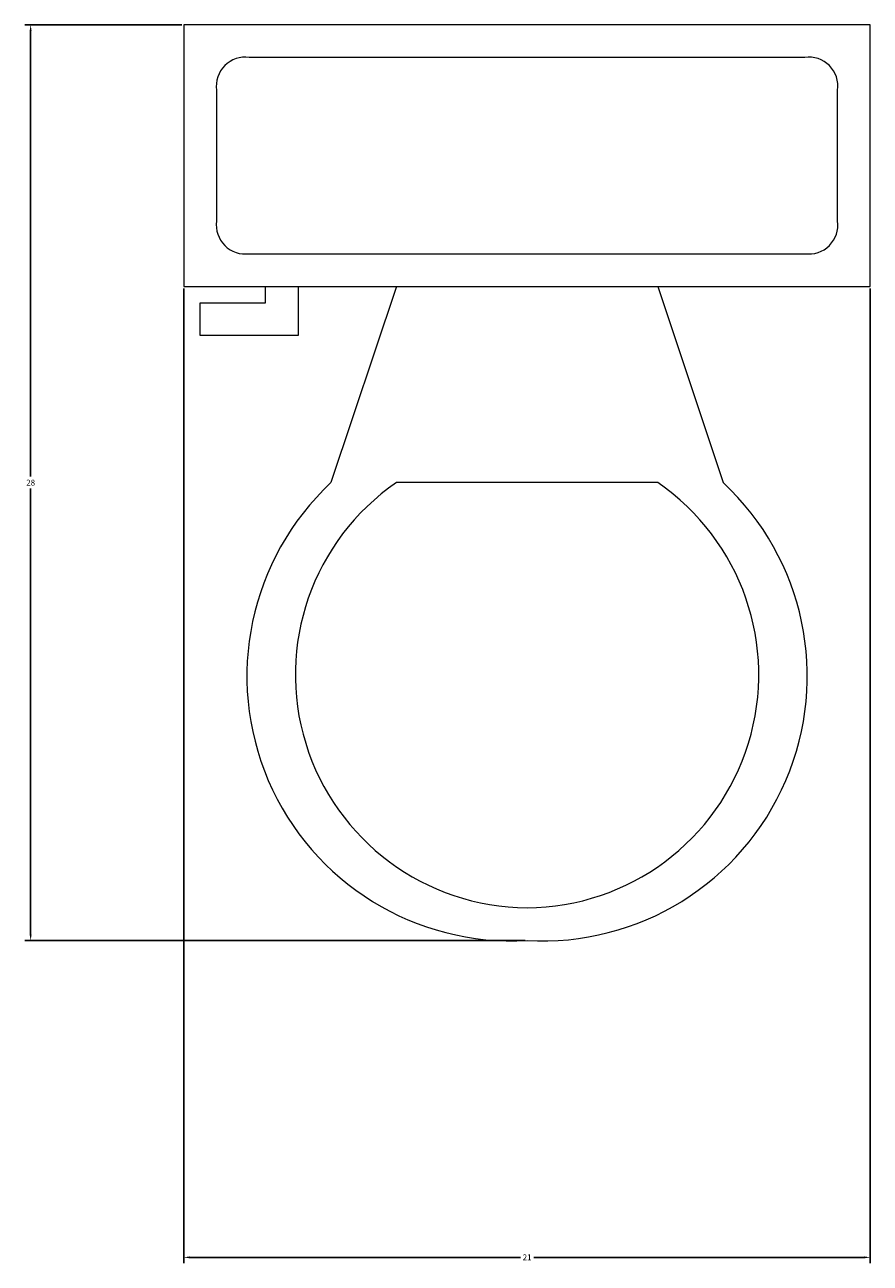
# Model space of a CAD drawing. Units: inches. Extents: x 2070 to 4408, y 1595 to 4269.
# Tile 20 of 20: x 4382 to 4408, y 4231 to 4269. Entities that reach past the tile are written whole.
import ezdxf

# ---------------------------------------------------------------- set-up
doc = ezdxf.new("R2010")
doc.units = ezdxf.units.IN
doc.layers.add('A-ANNO-DIMS', color=2, linetype='Continuous', lineweight=18)
doc.layers.add('A-FLOR-FIXT', color=9, linetype='Continuous', lineweight=18)
doc.styles.get("Standard").update_dxf_attribs({"font": 'arial.ttf'})
doc.dimstyles.get("Standard").update_dxf_attribs({"dimtxt": 0.18, "dimasz": 0.18, "dimexe": 0.18, "dimexo": 0.0625, "dimgap": 0.09, "dimtad": 0, "dimtih": 1, "dimtoh": 1, "dimdec": 4, "dimzin": 0, "dimdsep": 46, "dimtxsty": 'Standard', "dimcen": 0.09, "dimadec": 0, "dimazin": 0, "dimtfac": 1, "dimtdec": 4, "dimtofl": 0, "dimtmove": 0, "dimatfit": 3, "dimfxl": 1, "dimtolj": 1, "dimtzin": 0, "dimarcsym": 0})

# ---------------------------------------------------------------- blocks, each defined once
blk = doc.blocks.new('*U11')
for p, q in [((241.3, -152.4), (241.3, -50.8)), ((-203.2, -215.9), (-203.2, -203.2)), ((-177.8, -203.2), (-177.8, -241.3)), ((-101.6, -203.2), (-152.4, -355.6)), ((101.6, -203.2), (152.4, -355.6)), ((-254, -215.9), (-203.2, -215.9)), ((-254, -241.3), (-254, -215.9)), ((-177.8, -241.3), (-254, -241.3)), ((101.6, -355.6), (-101.6, -355.6))]:
    blk.add_line(p, q)
blk.add_lwpolyline([(266.7, -203.2), (266.7, 0), (-266.7, 0), (-266.7, -203.2)], close=True)
for points in [[(215.9, -25.4), (-215.9, -25.4)], [(-241.3, -50.8), (-241.3, -152.4)], [(-215.9, -177.8), (215.9, -177.8)]]:
    blk.add_lwpolyline(points)
for centre, radius, start, end in [((-219.075, -47.625), 22.45064, 81.8699, 188.1301), ((219.075, -47.625), 22.45064, 351.8699, 98.1301), ((-219.075, -155.575), 22.45064, 171.869898, 278.1301), ((219.075, -155.575), 22.45064, 261.8699, 8.1301), ((-12.12088, -505.93752), 205.61935, 133.01722, 273.38), ((0.94996, -504.77674), 181.02486, 124.50543, 269.7), ((-0.94742, -504.77674), 181.02486, 270.3, 55.4946), ((12.12342, -505.93752), 205.61935, 266.62, 46.9828)]:
    blk.add_arc(centre, radius, start, end)
blk = doc.blocks.new('*D43')
at = {"layer": 'A-ANNO-DIMS', "color": 0, "lineweight": -2, "transparency": 16777216}
for p, q in [((4387.185, 4260.818), (4387.185, 4231.01)), ((4408.185, 4260.818), (4408.185, 4231.01)), ((4387.365, 4231.19), (4397.482, 4231.19)), ((4408.005, 4231.19), (4397.888, 4231.19))]:
    blk.add_line(p, q, dxfattribs=at)
at = {"layer": 'A-ANNO-DIMS', "color": 0, "transparency": 16777216}
for points in [[(4387.365, 4231.22), (4387.365, 4231.16), (4387.185, 4231.19)], [(4408.005, 4231.22), (4408.005, 4231.16), (4408.185, 4231.19)]]:
    blk.add_solid(points, dxfattribs=at)
at = {"layer": 'Defpoints', "color": 0, "transparency": 16777216}
for p in [(4387.185, 4260.88), (4408.185, 4260.88), (4408.185, 4231.19)]:
    blk.add_point(p, dxfattribs=at)
at = {"layer": 'A-ANNO-DIMS', "color": 0, "transparency": 16777216, "insert": (4397.685, 4231.19), "char_height": 0.18, "attachment_point": 5}
blk.add_mtext('\\A1;21', dxfattribs=at)
blk = doc.blocks.new('*D44')
at = {"layer": 'A-ANNO-DIMS', "color": 0, "lineweight": -2, "transparency": 16777216}
for p, q in [((4387.122, 4268.88), (4382.315, 4268.88)), ((4382.495, 4268.7), (4382.495, 4255.062)), ((4382.495, 4241.06), (4382.495, 4254.698)), ((4397.622, 4240.88), (4382.315, 4240.88))]:
    blk.add_line(p, q, dxfattribs=at)
at = {"layer": 'A-ANNO-DIMS', "color": 0, "transparency": 16777216}
for points in [[(4382.465, 4268.7), (4382.525, 4268.7), (4382.495, 4268.88)], [(4382.465, 4241.06), (4382.525, 4241.06), (4382.495, 4240.88)]]:
    blk.add_solid(points, dxfattribs=at)
at = {"layer": 'Defpoints', "color": 0, "transparency": 16777216}
for p in [(4382.495, 4268.88), (4387.185, 4268.88), (4397.685, 4240.88)]:
    blk.add_point(p, dxfattribs=at)
at = {"layer": 'A-ANNO-DIMS', "color": 0, "transparency": 16777216, "insert": (4382.495, 4254.88), "char_height": 0.18, "attachment_point": 5}
blk.add_mtext('\\A1;28', dxfattribs=at)

msp = doc.modelspace()

# ---------------------------------------------------------------- block references
at = {"layer": 'A-FLOR-FIXT', "xscale": 0.0393700787401575, "yscale": 0.0393700787401575, "zscale": 0.0393700787401575}
msp.add_blockref('*U11', (4397.6846, 4268.8802), dxfattribs=at)

# ---------------------------------------------------------------- dimensions: what is measured, and where the dimension line sits
at = {"layer": 'A-ANNO-DIMS'}
dim = msp.add_linear_dim(base=(4382.4946, 4268.8802), p1=(4397.6847, 4240.8802), p2=(4387.1846, 4268.8802), angle=90, dimstyle='Standard', override={"dimdec": 0, "dimlfac": 1, "dimrnd": 0, "dimzin": 0, "dimdsep": 46, "dimlunit": 2}, dxfattribs=at)
dim.commit()
dim.dimension.update_dxf_attribs({"geometry": '*D44', "text_midpoint": (4382.4946, 4254.8802)})
dim = msp.add_linear_dim(base=(4408.1846, 4231.1902), p1=(4387.1846, 4260.8802), p2=(4408.1846, 4260.8802), dimstyle='Standard', override={"dimdec": 0, "dimlfac": 1, "dimrnd": 0, "dimzin": 0, "dimdsep": 46, "dimlunit": 2}, dxfattribs=at)
dim.commit()
dim.dimension.update_dxf_attribs({"geometry": '*D43', "text_midpoint": (4397.6846, 4231.1902)})

doc.saveas('drawing.dxf')
